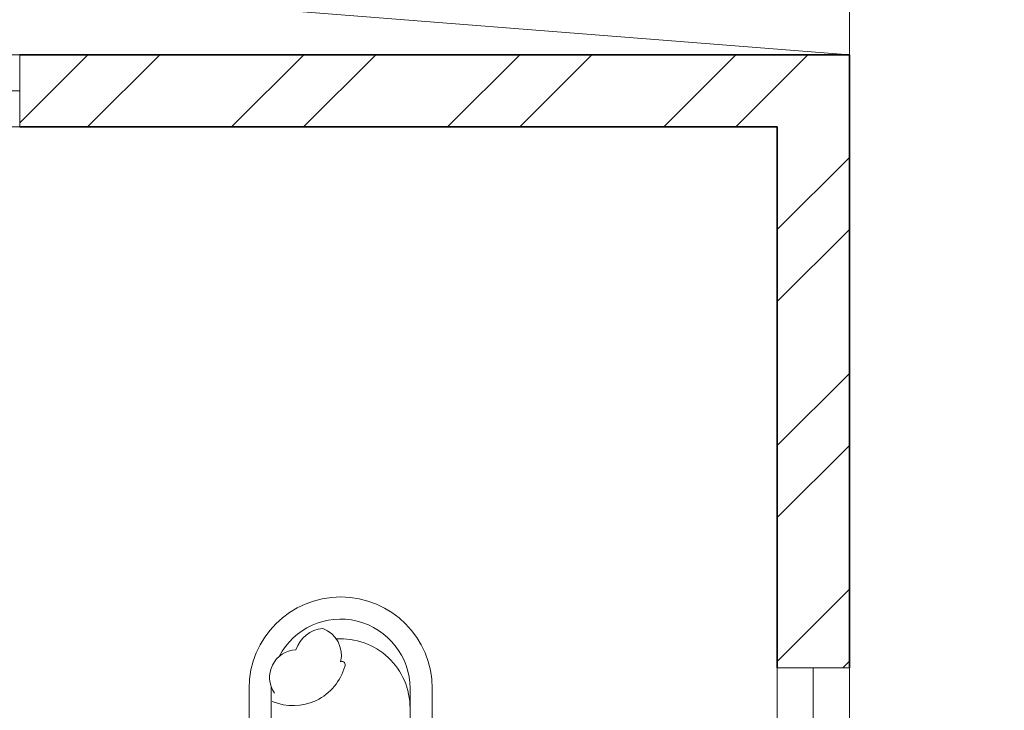
# Model space of a CAD drawing. Units: inches. Extents: x 1885 to 2748, y 783 to 2421.
# Tile 53 of 117: x 2396 to 2457, y 1807 to 1850. Entities that reach past the tile are written whole.
import ezdxf

# ---------------------------------------------------------------- set-up
doc = ezdxf.new("R2010")
doc.units = ezdxf.units.IN
for name, color, linetype, lineweight in [('A-FLOR-OPEN', 8, 'Continuous', 13), ('A-FURN', 8, 'Continuous', 13), ('A-GLAZ', 181, 'Continuous', 18), ('A-WALL', 7, 'Continuous', 35)]:
    doc.layers.add(name, color=color, linetype=linetype, lineweight=lineweight)
doc.layers.add('A-WALL-PATT', color=85, linetype='Continuous', lineweight=13, true_color=0x58ba48)

# ---------------------------------------------------------------- blocks, each defined once
blk = doc.blocks.new('CHAIR-LOUNGE')
blk.add_line((1.388, 5.701), (1.383, 10.98))
at = {"ltscale": 0.03}
blk.add_lwpolyline([(1.383, 10.98, 0.369229), (-0.002, 10.979), (0.003, 5.7, 1), (11.423, 5.711), (11.418, 10.99, 0.369229), (10.034, 10.988)], format="xyb", close=True, dxfattribs=at)
blk.add_lwpolyline([(1.877, 3.707, 0.785087), (10.039, 5.71), (10.034, 10.988)], format="xyb")
for centre, radius, start, end in [((2.748, 3.424), 3.35, 15.71431, 112.98573), ((5.712, 6.928), 4.326, 266.34198, 0.05385), ((3.014, 5.016), 1.734, 145.85992, 267.00778), ((5.713, 5.706), 4.326, 180.05385, 181.14637), ((5.792, 4.23), 0.207, 246.25768, 29.37621), ((3.979, 3.63), 1.778, 290.53054, 13.35968), ((4.772, 3.909), 1.951, 198.64662, 265.00007)]:
    blk.add_arc(centre, radius, start, end)
blk = doc.blocks.new('WIN-60')
for p, q in [((0.004, 59.998), (4.504, 59.998)), ((0.004, 59.998), (0.004, -0.002)), ((4.504, 59.998), (2.254, 59.998)), ((2.254, 59.998), (2.254, -0.002)), ((4.504, -0.002), (4.504, 59.998)), ((2.254, -0.002), (0.004, -0.002)), ((0.004, -0.002), (4.504, -0.002))]:
    blk.add_line(p, q)

msp = doc.modelspace()

# ---------------------------------------------------------------- hatches: boundary and pattern name
at = {"layer": 'A-WALL-PATT'}
h = msp.add_hatch(dxfattribs=at)
h.set_pattern_fill('ANSI32', color=256)
h.paths.add_polyline_path([(2007.772, 2318.006), (1980.774, 2318.006), (1980.774, 2281.215), (1985.274, 2281.215), (1985.274, 2313.506), (2007.772, 2313.506), (2007.772, 2315.756)])
h.paths.add_polyline_path([(2094.324, 2318.006), (2067.772, 2318.006), (2067.772, 2313.506), (2094.324, 2313.506), (2094.324, 2315.756)])
h.paths.add_polyline_path([(2131.367, 2315.756), (2131.367, 2318.006), (2131.189, 2318.006), (2112.609, 2318.006), (2112.609, 2313.506), (2117.274, 2313.506), (2117.274, 2255.201), (2121.774, 2255.201), (2121.774, 2313.506), (2131.367, 2313.506)])
h.paths.add_polyline_path([(2190.512, 2318.006), (2155.367, 2318.006), (2155.367, 2313.506), (2169.774, 2313.506), (2169.774, 2229.506), (2121.774, 2229.506), (2121.774, 2233.451), (2119.524, 2233.451), (2117.274, 2233.451), (2117.274, 2201.101), (2121.774, 2201.101), (2121.774, 2225.006), (2169.774, 2225.006), (2169.774, 2165.006), (2306.274, 2165.006), (2306.274, 2066.006), (2310.774, 2066.006), (2344.274, 2066.006), (2486.274, 2066.006), (2486.274, 1886.006), (2483.02, 1886.006), (2483.02, 1881.506), (2486.274, 1881.506), (2486.274, 1880.678), (2490.774, 1880.678), (2490.774, 2070.506), (2344.274, 2070.506), (2310.774, 2070.506), (2310.774, 2165.006), (2310.774, 2173.636), (2308.524, 2173.636), (2306.274, 2173.636), (2306.274, 2169.506), (2174.274, 2169.506), (2174.274, 2313.506), (2190.512, 2313.506), (2190.512, 2315.756)])
h.paths.add_polyline_path([(1985.274, 2221.215), (1980.774, 2221.215), (1980.774, 2165.006), (1992.774, 2165.006), (1992.774, 2141.927), (1997.274, 2141.927), (1997.274, 2165.006), (2117.274, 2165.006), (2117.274, 2163.126), (2121.774, 2163.126), (2121.774, 2172.734), (2119.524, 2172.734), (2117.274, 2172.734), (2117.274, 2169.506), (1985.274, 2169.506)])
h.paths.add_polyline_path([(1997.274, 2105.927), (1992.774, 2105.927), (1992.774, 2070.506), (2016.774, 2070.506), (2016.774, 2059.123), (2019.024, 2059.123), (2021.274, 2059.123), (2021.274, 2070.506), (2117.274, 2070.506), (2117.274, 2022.506), (2114.423, 2022.506), (2114.423, 2018.006), (2123.627, 2018.006), (2123.627, 2020.256), (2123.627, 2022.506), (2121.774, 2022.506), (2121.774, 2142.587), (2119.524, 2142.587), (2117.274, 2142.587), (2117.274, 2075.006), (1997.274, 2075.006)])
h.paths.add_polyline_path([(2092.029, 2020.256), (2092.029, 2022.506), (2021.274, 2022.506), (2021.274, 2035.123), (2016.774, 2035.123), (2016.774, 2018.006), (2016.774, 1978.784), (2021.274, 1978.784), (2021.274, 2018.006), (2092.029, 2018.006)])
h.paths.add_polyline_path([(2260.938, 2022.506), (2153.105, 2022.506), (2153.105, 2020.256), (2153.105, 2018.006), (2155.274, 2018.006), (2155.274, 1886.006), (2107.629, 1886.006), (2107.629, 1881.506), (2182.911, 1881.506), (2182.911, 1883.756), (2182.911, 1886.006), (2159.774, 1886.006), (2159.774, 2018.006), (2260.938, 2018.006), (2260.938, 2020.256)])
h.paths.add_polyline_path([(2047.629, 1883.756), (2047.629, 1886.006), (2021.274, 1886.006), (2021.274, 1918.784), (2019.024, 1918.784), (2016.774, 1918.784), (2016.774, 1881.506), (2047.629, 1881.506)])
h.paths.add_polyline_path([(2306.361, 1883.756), (2306.361, 1886.006), (2296.274, 1886.006), (2296.274, 1982.006), (2316.535, 1982.006), (2316.535, 1984.256), (2316.535, 1986.506), (2296.274, 1986.506), (2296.274, 2022.506), (2289.276, 2022.506), (2289.276, 2018.006), (2291.774, 2018.006), (2291.774, 1886.006), (2242.911, 1886.006), (2242.911, 1881.506), (2306.361, 1881.506)], flags=17)
h.paths.add_polyline_path([(1985.274, 1843.006), (2021.6, 1843.006), (2021.534, 1845.441), (2021.477, 1847.506), (1980.774, 1847.506), (1980.774, 1809.446), (1985.274, 1809.446)])
h.paths.add_polyline_path([(2131.482, 1845.256), (2131.482, 1847.506), (2081.534, 1847.506), (2081.534, 1843.006), (2117.274, 1843.006), (2117.274, 1784.147), (2119.524, 1784.147), (2121.774, 1784.147), (2121.774, 1843.006), (2131.482, 1843.006)])
h.paths.add_polyline_path([(2203.886, 1847.506), (2155.482, 1847.506), (2155.482, 1843.006), (2169.774, 1843.006), (2169.774, 1759.006), (2121.774, 1759.006), (2121.774, 1761.457), (2117.274, 1761.457), (2117.274, 1730.429), (2121.774, 1730.429), (2121.774, 1754.506), (2177.421, 1754.506), (2177.421, 1756.756), (2177.421, 1759.006), (2174.274, 1759.006), (2174.274, 1843.006), (2203.886, 1843.006)])
h.paths.add_polyline_path([(2335.554, 1845.256), (2335.554, 1847.506), (2239.886, 1847.506), (2239.886, 1843.006), (2306.274, 1843.006), (2306.274, 1759.006), (2199.486, 1759.006), (2199.486, 1754.506), (2310.774, 1754.506), (2310.774, 1843.006), (2335.554, 1843.006)])
h.paths.add_polyline_path([(2348.774, 2022.506), (2344.274, 2022.506), (2344.274, 1986.506), (2341.681, 1986.506), (2341.681, 1982.006), (2344.274, 1982.006), (2344.274, 1886.006), (2330.361, 1886.006), (2330.361, 1881.506), (2361.627, 1881.506), (2361.627, 1883.756), (2361.627, 1886.006), (2348.774, 1886.006)], flags=17)
h.paths.add_polyline_path([(2283.251, 2315.756), (2283.251, 2318.006), (2238.512, 2318.006), (2238.512, 2313.506), (2283.251, 2313.506)], flags=17)
h.paths.add_polyline_path([(2363.274, 2348.006), (2388.677, 2348.006), (2388.677, 2350.256), (2388.677, 2352.506), (2358.774, 2352.506), (2358.774, 2348.006), (2358.774, 2318.006), (2344.481, 2318.006), (2344.481, 2313.506), (2358.774, 2313.506), (2358.774, 2229.506), (2310.774, 2229.506), (2310.774, 2231.952), (2306.274, 2231.952), (2306.274, 2205.611), (2310.774, 2205.611), (2310.774, 2225.006), (2358.774, 2225.006), (2358.774, 2211.506), (2452.329, 2211.506), (2452.329, 2213.756), (2452.329, 2216.006), (2363.274, 2216.006), (2363.274, 2318.006)])
h.paths.add_polyline_path([(2310.774, 2313.506), (2320.481, 2313.506), (2320.481, 2315.756), (2320.481, 2318.006), (2302.728, 2318.006), (2302.728, 2313.506), (2306.274, 2313.506), (2306.274, 2251.076), (2310.774, 2251.076)], flags=17)
h.paths.add_polyline_path([(2490.774, 2352.506), (2486.274, 2352.506), (2448.677, 2352.506), (2448.677, 2348.006), (2486.274, 2348.006), (2486.274, 2318.006), (2486.274, 2216.006), (2481.78, 2216.006), (2481.78, 2211.506), (2486.274, 2211.506), (2486.274, 2165.006), (2493.289, 2165.006), (2493.289, 2167.256), (2493.289, 2169.506), (2490.774, 2169.506), (2490.774, 2313.506), (2494.429, 2313.506), (2494.429, 2318.006), (2490.774, 2318.006)])
h.paths.add_polyline_path([(2534.653, 2318.006), (2515.691, 2318.006), (2515.691, 2313.506), (2534.653, 2313.506), (2534.653, 2315.756)])
h.paths.add_polyline_path([(2618.274, 2318.006), (2594.653, 2318.006), (2594.653, 2313.506), (2613.774, 2313.506), (2613.774, 2281.706), (2618.274, 2281.706)])
h.paths.add_polyline_path([(2618.274, 2221.706), (2613.774, 2221.706), (2613.774, 2169.506), (2554.019, 2169.506), (2554.019, 2165.006), (2613.774, 2165.006), (2613.774, 2152.878), (2618.274, 2152.878)])
h.paths.add_polyline_path([(2618.274, 2128.878), (2616.024, 2128.878), (2613.774, 2128.878), (2613.774, 2117.006), (2529.774, 2117.006), (2529.774, 2165.006), (2532.848, 2165.006), (2532.848, 2169.506), (2522.867, 2169.506), (2522.867, 2165.006), (2525.274, 2165.006), (2525.274, 2117.006), (2525.274, 2112.506), (2525.274, 2108.576), (2529.774, 2108.576), (2529.774, 2112.506), (2613.774, 2112.506), (2613.774, 2080.19), (2618.274, 2080.19)])
h.paths.add_polyline_path([(2618.274, 2044.19), (2616.024, 2044.19), (2613.774, 2044.19), (2613.774, 2015.506), (2529.774, 2015.506), (2529.774, 2088.582), (2527.524, 2088.582), (2525.274, 2088.582), (2525.274, 2011.006), (2613.774, 2011.006), (2613.774, 1956.755), (2618.274, 1956.755)])
h.paths.add_polyline_path([(2618.274, 1881.506), (2618.274, 1896.755), (2613.774, 1896.755), (2613.774, 1881.506), (2613.774, 1847.506), (2592.715, 1847.506), (2592.715, 1843.006), (2613.774, 1843.006), (2613.774, 1765.006), (2613.774, 1760.506), (2609.621, 1760.506), (2609.621, 1756.006), (2613.774, 1756.006), (2613.774, 1660.006), (2608.544, 1660.006), (2608.544, 1655.506), (2613.774, 1655.506), (2613.774, 1508.158), (2618.274, 1508.158)])
h.paths.add_polyline_path([(2565.774, 1843.006), (2568.997, 1843.006), (2568.997, 1847.506), (2490.774, 1847.506), (2490.774, 1849.7), (2488.524, 1849.7), (2486.274, 1849.7), (2486.274, 1847.506), (2477.274, 1847.506), (2477.274, 1838.506), (2477.274, 1821.493), (2486.274, 1821.493), (2486.274, 1838.506), (2561.274, 1838.506), (2561.274, 1765.006), (2486.274, 1765.006), (2486.274, 1786.157), (2477.274, 1786.157), (2477.274, 1765.006), (2477.274, 1756.006), (2486.274, 1756.006), (2565.774, 1756.006), (2585.621, 1756.006), (2585.621, 1758.256), (2585.621, 1760.506), (2565.774, 1760.506), (2565.774, 1765.006)])
h.paths.add_polyline_path([(2486.274, 1651.006), (2561.274, 1651.006), (2561.274, 1567.006), (2486.274, 1567.006), (2486.274, 1591.321), (2477.274, 1591.321), (2477.274, 1567.006), (2477.274, 1558.006), (2477.274, 1555.439), (2481.774, 1555.439), (2481.774, 1558.006), (2568.653, 1558.006), (2568.653, 1560.256), (2568.653, 1562.506), (2565.774, 1562.506), (2565.774, 1655.506), (2584.544, 1655.506), (2584.544, 1657.756), (2584.544, 1660.006), (2565.774, 1660.006), (2486.274, 1660.006), (2477.274, 1660.006), (2477.274, 1651.006), (2477.274, 1632.989), (2486.274, 1632.989)])
h.paths.add_polyline_path([(2449.967, 1883.756), (2449.967, 1886.006), (2421.627, 1886.006), (2421.627, 1881.506), (2449.967, 1881.506)], flags=17)
h.paths.add_polyline_path([(2447.274, 1847.506), (2395.554, 1847.506), (2395.554, 1843.006), (2442.774, 1843.006), (2442.774, 1809.27), (2447.274, 1809.27)])
h.paths.add_polyline_path([(1985.274, 1749.446), (1980.774, 1749.446), (1980.774, 1694.504), (1985.274, 1694.504), (1985.274, 1694.506), (1986.897, 1694.506), (1986.897, 1697.78), (1986.897, 1699.006), (1985.274, 1699.006)])
h.paths.add_polyline_path([(2152.774, 1699.006), (2121.774, 1699.006), (2121.774, 1703.668), (2119.524, 1703.668), (2117.274, 1703.668), (2117.274, 1699.006), (2009.219, 1699.006), (2009.219, 1694.506), (2148.274, 1694.506), (2148.274, 1692.631), (2152.774, 1692.631)])
h.paths.add_polyline_path([(2016.274, 1694.506), (2011.774, 1694.506), (2011.774, 1558.006), (2040.806, 1558.006), (2040.806, 1560.256), (2040.806, 1562.506), (2016.274, 1562.506)])
h.paths.add_polyline_path([(2152.774, 1663.017), (2150.524, 1663.017), (2148.274, 1663.017), (2148.274, 1562.506), (2100.806, 1562.506), (2100.806, 1558.006), (2165.119, 1558.006), (2165.119, 1560.256), (2165.119, 1562.506), (2152.774, 1562.506), (2152.774, 1610.506), (2224.774, 1610.506), (2224.774, 1607.99), (2229.274, 1607.99), (2229.274, 1615.006), (2152.774, 1615.006)])
h.paths.add_polyline_path([(2238.613, 1560.256), (2238.613, 1562.506), (2229.274, 1562.506), (2229.274, 1588.756), (2227.024, 1588.763), (2224.774, 1588.771), (2224.774, 1562.506), (2189.119, 1562.506), (2189.119, 1558.006), (2238.613, 1558.006)])
h.paths.add_polyline_path([(2336.024, 1560.256), (2336.024, 1562.506), (2310.774, 1562.506), (2310.774, 1656.347), (2308.524, 1656.347), (2306.274, 1656.347), (2306.274, 1562.506), (2286.613, 1562.506), (2286.613, 1558.006), (2336.024, 1558.006)])
h.paths.add_polyline_path([(2447.274, 1690.968), (2445.024, 1690.968), (2442.774, 1690.968), (2442.774, 1687.006), (2306.274, 1687.006), (2306.274, 1680.75), (2310.774, 1680.75), (2310.774, 1682.506), (2442.774, 1682.506), (2442.774, 1562.506), (2396.024, 1562.506), (2396.024, 1558.006), (2447.274, 1558.006)])
h.paths.add_polyline_path([(2447.274, 1749.27), (2445.024, 1749.27), (2442.774, 1749.27), (2442.774, 1717.232), (2447.274, 1717.232)])
h.paths.add_polyline_path([(2044.674, 1521.756), (2044.674, 1524.006), (2007.274, 1524.006), (2007.274, 1503.49), (2009.524, 1503.49), (2011.774, 1503.49), (2011.774, 1519.506), (2044.674, 1519.506)])
h.paths.add_polyline_path([(2177.969, 1521.756), (2177.969, 1524.006), (2104.674, 1524.006), (2104.674, 1519.506), (2145.774, 1519.506), (2145.774, 1387.506), (2143.37, 1387.506), (2143.37, 1383.006), (2251.585, 1383.006), (2251.585, 1385.256), (2251.585, 1387.506), (2150.274, 1387.506), (2150.274, 1519.506), (2177.969, 1519.506)])
h.paths.add_polyline_path([(2298.704, 1524.006), (2237.969, 1524.006), (2237.969, 1519.506), (2282.274, 1519.506), (2282.274, 1387.506), (2279.683, 1387.506), (2279.683, 1383.006), (2286.774, 1383.006), (2286.774, 1419.006), (2312.451, 1419.006), (2312.451, 1421.256), (2312.451, 1423.506), (2286.774, 1423.506), (2286.774, 1519.506), (2298.704, 1519.506), (2298.704, 1521.722)], flags=17)
h.paths.add_polyline_path([(2361.897, 1521.756), (2361.897, 1524.006), (2322.704, 1524.006), (2322.704, 1519.506), (2334.774, 1519.506), (2334.774, 1423.506), (2331.93, 1423.506), (2331.93, 1419.006), (2334.774, 1419.006), (2334.774, 1387.506), (2334.774, 1383.228), (2339.274, 1383.228), (2339.274, 1387.506), (2339.274, 1519.506), (2361.897, 1519.506)], flags=17)
h.paths.add_polyline_path([(2447.274, 1521.756), (2447.274, 1524.006), (2421.897, 1524.006), (2421.897, 1519.506), (2447.274, 1519.506)], flags=17)
h.paths.add_polyline_path([(2481.774, 1529.6), (2479.524, 1529.6), (2477.274, 1529.6), (2477.274, 1524.006), (2474.489, 1524.006), (2474.489, 1519.506), (2477.274, 1519.506), (2477.274, 1334.506), (2296.774, 1334.506), (2296.774, 1240.506), (2160.274, 1240.506), (2160.274, 1180.506), (2112.274, 1180.506), (2112.274, 1207.692), (2110.024, 1207.692), (2107.774, 1207.692), (2107.774, 1171.609), (2112.274, 1171.609), (2112.274, 1176.006), (2160.274, 1176.006), (2160.274, 1092.006), (2144.221, 1092.006), (2144.221, 1087.506), (2189.497, 1087.506), (2189.497, 1089.756), (2189.497, 1092.006), (2164.774, 1092.006), (2164.774, 1236.006), (2296.774, 1236.006), (2296.774, 1231.912), (2301.274, 1231.912), (2301.274, 1330.006), (2481.774, 1330.006), (2481.774, 1387.506)])
h.paths.add_polyline_path([(2618.274, 1448.158), (2613.774, 1448.158), (2613.774, 1382.506), (2529.774, 1382.506), (2525.274, 1382.506), (2525.274, 1307.062), (2529.774, 1307.062), (2529.774, 1378.006), (2613.774, 1378.006), (2613.774, 1354.988), (2618.274, 1354.988)])
h.paths.add_polyline_path([(2618.274, 1318.988), (2613.774, 1318.988), (2613.774, 1281.006), (2529.774, 1281.006), (2529.774, 1283.786), (2527.524, 1283.786), (2525.274, 1283.786), (2525.274, 1228.506), (2516.794, 1228.506), (2516.794, 1224.006), (2533.484, 1224.006), (2533.484, 1226.256), (2533.484, 1228.506), (2529.774, 1228.506), (2529.774, 1276.506), (2613.774, 1276.506), (2613.774, 1266.02), (2618.274, 1266.02)])
h.paths.add_polyline_path([(2618.274, 1134.964), (2613.774, 1134.964), (2613.774, 1092.006), (2594.545, 1092.006), (2594.545, 1087.506), (2618.274, 1087.506)])
h.paths.add_polyline_path([(2534.545, 1092.006), (2509.765, 1092.006), (2509.765, 1087.506), (2534.545, 1087.506), (2534.545, 1089.756)])
h.paths.add_polyline_path([(2481.274, 1224.006), (2484.117, 1224.006), (2484.117, 1226.256), (2484.117, 1228.506), (2476.774, 1228.506), (2476.774, 1198.506), (2471.61, 1198.506), (2471.61, 1194.006), (2476.774, 1194.006), (2476.774, 1062.006), (2436.894, 1062.006), (2436.894, 1057.506), (2476.774, 1057.506), (2481.274, 1057.506), (2481.274, 1062.006), (2481.274, 1087.506), (2485.354, 1087.506), (2485.354, 1089.756), (2485.354, 1092.006), (2481.274, 1092.006), (2481.274, 1117.506)])
h.paths.add_polyline_path([(2439.898, 1198.506), (2349.274, 1198.506), (2349.274, 1194.006), (2349.274, 1180.506), (2301.274, 1180.506), (2301.274, 1201.896), (2299.024, 1201.896), (2296.774, 1201.896), (2296.774, 1172.335), (2299.024, 1172.335), (2301.274, 1172.335), (2301.274, 1176.006), (2349.274, 1176.006), (2349.274, 1092.006), (2334.452, 1092.006), (2334.452, 1087.506), (2349.274, 1087.506), (2349.274, 1057.506), (2353.774, 1057.506), (2376.894, 1057.506), (2376.894, 1059.756), (2376.894, 1062.006), (2353.774, 1062.006), (2353.774, 1087.506), (2353.774, 1180.506), (2353.774, 1194.006), (2439.898, 1194.006), (2439.898, 1196.256)])
h.paths.add_polyline_path([(2270.596, 1089.756), (2270.596, 1092.006), (2249.497, 1092.006), (2249.497, 1087.506), (2270.596, 1087.506)], flags=17)
h.paths.add_polyline_path([(2310.452, 1092.006), (2301.274, 1092.006), (2301.274, 1153.292), (2296.774, 1153.292), (2296.774, 1092.006), (2293.786, 1092.006), (2293.786, 1087.506), (2310.452, 1087.506), (2310.452, 1089.756)], flags=17)
h.paths.add_polyline_path([(2112.274, 1150.328), (2110.024, 1150.328), (2107.774, 1150.328), (2107.774, 1092.006), (2104.465, 1092.006), (2104.465, 1087.506), (2120.221, 1087.506), (2120.221, 1089.756), (2120.221, 1092.006), (2112.274, 1092.006)])
h.paths.add_polyline_path([(2082.172, 1092.006), (2058.144, 1092.006), (2058.144, 1087.506), (2082.172, 1087.506), (2082.172, 1089.756)])
h.paths.add_polyline_path([(1975.774, 1145.638), (1971.274, 1145.638), (1971.274, 1087.506), (1980.774, 1087.506), (1998.144, 1087.506), (1998.144, 1089.756), (1998.144, 1092.006), (1985.274, 1092.006), (1975.774, 1092.006)])
h.paths.add_polyline_path([(2112.274, 1244.385), (2110.024, 1244.385), (2107.774, 1244.385), (2107.774, 1240.506), (1992.274, 1240.506), (1992.274, 1271.008), (1987.774, 1271.008), (1987.774, 1240.506), (1980.774, 1240.506), (1975.774, 1240.506), (1971.274, 1240.506), (1971.274, 1205.638), (1975.774, 1205.638), (1975.774, 1236.006), (2107.774, 1236.006), (2107.774, 1233.444), (2112.274, 1233.444), (2112.274, 1236.006)])
h.paths.add_polyline_path([(2112.274, 1383.006), (2114.783, 1383.006), (2114.783, 1385.256), (2114.783, 1387.506), (2102.476, 1387.506), (2102.476, 1383.006), (2107.774, 1383.006), (2107.774, 1335.006), (2011.774, 1335.006), (2011.774, 1349.939), (2007.274, 1349.939), (2007.274, 1335.006), (1987.774, 1335.006), (1987.774, 1330.506), (1987.774, 1307.008), (1992.274, 1307.008), (1992.274, 1330.506), (2007.274, 1330.506), (2107.774, 1330.506), (2107.774, 1264.711), (2112.274, 1264.711)])
h.paths.add_polyline_path([(2077.857, 1387.506), (2011.774, 1387.506), (2011.774, 1390.036), (2009.524, 1390.036), (2007.274, 1390.036), (2007.274, 1373.939), (2011.774, 1373.939), (2011.774, 1383.006), (2077.857, 1383.006)])
h.paths.add_polyline_path([(2011.774, 1443.49), (2007.274, 1443.49), (2007.274, 1410.248), (2011.774, 1410.248)])

# ---------------------------------------------------------------- linework, layer by layer
at = {"layer": 'A-FLOR-OPEN'}
for q in [(2016.774, 1881.506), (2447.274, 1881.506)]:
    msp.add_line((2447.274, 1847.506), q, dxfattribs=at)
at = {"layer": 'A-WALL'}
for p, q in [((2395.554, 1847.506), (2447.274, 1847.506)), ((2447.274, 1847.506), (2447.274, 1809.27)), ((2395.554, 1843.006), (2442.774, 1843.006)), ((2442.774, 1843.006), (2442.774, 1809.27))]:
    msp.add_line(p, q, dxfattribs=at)

# ---------------------------------------------------------------- block references
at = {"layer": 'A-FURN', "extrusion": (0, 0, -1), "zscale": -1, "rotation": 180}
msp.add_blockref('CHAIR-LOUNGE', (-2409.85, 1813.682), dxfattribs=at)
at = {"layer": 'A-GLAZ', "extrusion": (0, 0, -1), "zscale": -1}
for p, rotation in [((-2335.556, 1843.002), 90), ((-2442.77, 1809.268), 180)]:
    msp.add_blockref('WIN-60', p, dxfattribs=dict(at, rotation=rotation))

doc.saveas('drawing.dxf')
